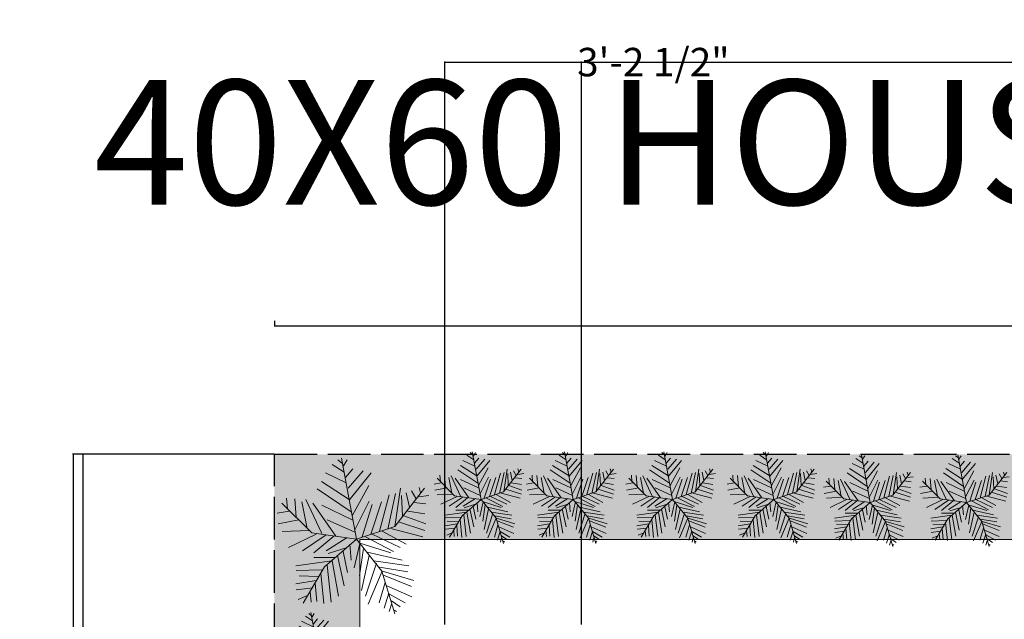
# Model space of a CAD drawing. Units: inches. Extents: x 853 to 1550, y 485 to 1596.
# Tile 14 of 18: x 862 to 1139, y 1428 to 1596. Entities that reach past the tile are written whole.
import ezdxf

# ---------------------------------------------------------------- set-up
doc = ezdxf.new("R2010")
doc.units = ezdxf.units.IN
doc.header["$MEASUREMENT"] = 0
doc.linetypes.add('ACAD_ISO02W100', pattern=[15, 12, -3])
for name, color, linetype, lineweight in [('A-ANNO-DIMS', 2, 'Continuous', 18), ('A-ANNO-TEXT', 250, 'Continuous', 25), ('C-PROP', 8, 'ACAD_ISO02W100', 25), ('L-PLNT-TREE', 106, 'Continuous', 13), ('lawn', 106, 'Continuous', 18)]:
    doc.layers.add(name, color=color, linetype=linetype, lineweight=lineweight)
doc.layers.add('L-PLNT-PATT', color=85, linetype='Continuous', lineweight=13, true_color=0x58ba48)
doc.styles.get("Standard").update_dxf_attribs({"font": 'arial.ttf'})
doc.dimstyles.get("Standard").update_dxf_attribs({"dimtxt": 8, "dimasz": 0.18, "dimexe": 0.18, "dimexo": 0.0625, "dimgap": 0.09, "dimtad": 0, "dimtih": 1, "dimtoh": 1, "dimzin": 0, "dimdsep": 46, "dimlunit": 3, "dimtxsty": 'Standard', "dimcen": 0.09, "dimadec": 0, "dimazin": 0, "dimtfac": 1, "dimtofl": 0, "dimtmove": 0, "dimatfit": 3, "dimfxl": 1, "dimtolj": 1, "dimtzin": 0, "dimarcsym": 0})

# ---------------------------------------------------------------- blocks, each defined once
blk = doc.blocks.new('*U18')
for p, q in [((-10.186, 53.64), (-13.084, 55.962)), ((0, 0), (-10.5, 57)), ((-9.099, 51.782), (-6.563, 55.962)), ((-8.737, 47.138), (-17.069, 52.711)), ((-7.65, 43.423), (-2.578, 49.46)), ((-7.288, 39.707), (-21.778, 46.673)), ((-5.839, 35.992), (4.667, 48.067)), ((-5.114, 27.632), (10.463, 46.673)), ((-3.665, 19.273), (-27.574, 35.527)), ((-5.114, 28.097), (-24.676, 40.636)), ((-2.941, 16.486), (8.652, 37.85)), ((27, 9), (48, 36)), ((27.127, 9.056), (31.112, 35.992)), ((44.153, 36.456), (45.239, 32.741)), ((-48.585, 21.131), (-49.309, 29.026)), ((-43.513, 28.561), (-42.427, 15.558)), ((-35.544, 28.097), (-24.314, 3.947)), ((16.259, 5.805), (23.142, 31.348)), ((22.055, 7.198), (27.489, 32.277)), ((31.836, 30.883), (32.561, 16.486)), ((35.096, 32.741), (37.27, 22.524)), ((38.719, 34.134), (41.979, 28.561)), ((43.791, 29.954), (51.036, 30.883)), ((-31.5, 4.5), (-52.5, 25.5)), ((-38.442, 26.239), (-34.819, 7.663)), ((-14.533, 2.09), (-30.834, 25.31)), ((-24.314, 23.917), (-2.941, 13.7)), ((-1.129, 6.734), (9.014, 26.704)), ((3.942, 1.625), (11.187, 24.381)), ((10.101, 3.483), (17.708, 26.239)), ((40.53, 25.775), (48.862, 24.846)), ((-47.498, 19.737), (-55.83, 18.344)), ((33.285, 16.486), (48.862, 10.913)), ((36.183, 19.737), (48.137, 17.88)), ((-40.615, 13.7), (-55.105, 10.913)), ((-20.691, 13.7), (-1.129, 4.876)), ((0, 0), (27, 9)), ((24.229, 7.663), (46.688, 1.625)), ((29.662, 12.307), (48.137, 6.269)), ((-33.37, 6.269), (-52.207, 5.34)), ((-28.299, 3.483), (-47.86, -5.805)), ((-21.416, 3.018), (-38.079, -8.128)), ((0, 0), (-31.5, 4.5)), ((-15.982, 2.09), (-30.11, -9.521)), ((0, 0), (-22.5, -19.5)), ((-6.563, 1.161), (-21.416, -8.128)), ((0, 0), (18, -22.5)), ((6.478, 1.625), (26.04, -8.592)), ((11.187, 3.483), (30.749, -5.805)), ((18.07, 5.805), (35.096, -3.483)), ((-6.563, -5.805), (-19.967, -9.985)), ((-4.752, -3.483), (-3.665, -14.629)), ((2.493, -3.019), (-1.491, -20.202)), ((1.769, -2.555), (24.229, -9.521)), ((5.029, -6.27), (2.131, -25.775)), ((-15.257, -12.772), (-30.11, -12.772)), ((-13.446, -11.378), (-8.737, -32.741)), ((-9.461, -8.592), (-6.201, -23.453)), ((9.014, -11.378), (3.58, -35.992)), ((7.565, -9.056), (32.198, -14.629)), ((-17.431, -15.094), (-42.789, -18.809)), ((-22.5, -19.5), (-37.5, -45)), ((-20.691, -18.345), (-17.793, -44.352)), ((-17.069, -15.094), (-12.721, -40.172)), ((14.085, -16.951), (6.478, -40.172)), ((12.274, -15.094), (36.907, -18.809)), ((16.259, -19.738), (36.183, -22.989)), ((-24.314, -21.596), (-42.427, -22.06)), ((-26.849, -26.24), (-40.253, -25.775)), ((-25.038, -23.918), (-22.865, -45.281)), ((18.07, -22.524), (8.289, -45.745)), ((18, -22.5), (27, -52.5)), ((18.433, -22.524), (40.53, -29.026)), ((19.157, -25.311), (38.719, -33.206)), ((-28.299, -29.026), (-42.789, -31.348)), ((-30.834, -34.135), (-42.427, -35.528)), ((-29.023, -30.884), (-27.936, -43.887)), ((20.244, -30.419), (15.897, -44.816)), ((21.331, -32.741), (39.081, -40.636)), ((-34.457, -39.708), (-40.978, -42.494)), ((-32.646, -36.921), (-31.921, -44.352)), ((22.78, -37.85), (19.519, -48.532)), ((22.78, -38.314), (34.372, -44.816)), ((24.591, -45.745), (23.142, -50.854)), ((24.591, -43.423), (30.749, -47.603)), ((26.764, -49.925), (28.213, -50.854))]:
    blk.add_line(p, q)
blk = doc.blocks.new('*D22')
at = {"layer": 'A-ANNO-DIMS', "color": 0, "lineweight": -2, "transparency": 16777216}
for p, q in [((933.94, 1511.65), (933.94, 1510.09)), ((1461.94, 1511.65), (1461.94, 1510.09)), ((934.12, 1510.27), (1190.9, 1510.27)), ((1461.76, 1510.27), (1204.98, 1510.27))]:
    blk.add_line(p, q, dxfattribs=at)
at = {"layer": 'A-ANNO-DIMS', "color": 0, "transparency": 16777216}
for points in [[(934.12, 1510.3), (934.12, 1510.24), (933.94, 1510.27)], [(1461.76, 1510.3), (1461.76, 1510.24), (1461.94, 1510.27)]]:
    blk.add_solid(points, dxfattribs=at)
at = {"layer": 'Defpoints', "color": 0, "transparency": 16777216}
for p in [(933.94, 1511.71), (1461.94, 1511.71), (1461.94, 1510.27)]:
    blk.add_point(p, dxfattribs=at)
at = {"layer": 'A-ANNO-DIMS', "color": 0, "transparency": 16777216, "insert": (1197.94, 1510.27), "char_height": 8, "attachment_point": 5}
blk.add_mtext("\\A1;40'", dxfattribs=at)
blk = doc.blocks.new('*D23')
at = {"layer": 'A-ANNO-DIMS', "color": 0, "lineweight": -2, "transparency": 16777216}
for p, q in [((879.97, 1474.13), (879.75, 1474.13)), ((879.93, 1473.95), (879.93, 1049.11)), ((879.93, 615.92), (879.93, 1040.76)), ((879.97, 615.74), (879.75, 615.74))]:
    blk.add_line(p, q, dxfattribs=at)
at = {"layer": 'A-ANNO-DIMS', "color": 0, "transparency": 16777216}
for points in [[(879.9, 1473.95), (879.96, 1473.95), (879.93, 1474.13)], [(879.9, 615.92), (879.96, 615.92), (879.93, 615.74)]]:
    blk.add_solid(points, dxfattribs=at)
at = {"layer": 'Defpoints', "color": 0, "transparency": 16777216}
for p in [(880.03, 1474.13), (879.93, 615.74), (880.03, 615.74)]:
    blk.add_point(p, dxfattribs=at)
at = {"layer": 'A-ANNO-DIMS', "color": 0, "transparency": 16777216, "insert": (879.93, 1044.94), "char_height": 8, "attachment_point": 5}
blk.add_mtext("\\A1;60'", dxfattribs=at)
blk = doc.blocks.new('*D69')
at = {"layer": 'A-ANNO-DIMS', "color": 0, "lineweight": -2, "transparency": 16777216}
for p, q in [((981.94, 1426.19), (981.94, 1584.65)), ((982.12, 1584.47), (1184.11, 1584.47)), ((1413.76, 1584.47), (1211.77, 1584.47)), ((1413.94, 1426.19), (1413.94, 1584.65))]:
    blk.add_line(p, q, dxfattribs=at)
at = {"layer": 'A-ANNO-DIMS', "color": 0, "transparency": 16777216}
for points in [[(982.12, 1584.5), (982.12, 1584.44), (981.94, 1584.47)], [(1413.76, 1584.5), (1413.76, 1584.44), (1413.94, 1584.47)]]:
    blk.add_solid(points, dxfattribs=at)
at = {"layer": 'Defpoints', "color": 0, "transparency": 16777216}
for p in [(1413.94, 1584.47), (981.94, 1426.13), (1413.94, 1426.13)]:
    blk.add_point(p, dxfattribs=at)
at = {"layer": 'A-ANNO-DIMS', "color": 0, "transparency": 16777216, "insert": (1197.94, 1584.47), "char_height": 8, "attachment_point": 5}
blk.add_mtext('\\A1;36\'-0"', dxfattribs=at)
blk = doc.blocks.new('*D71')
at = {"layer": 'A-ANNO-DIMS', "color": 0, "lineweight": -2, "transparency": 16777216}
for p, q in [((933.87, 1474.13), (877.09, 1474.13)), ((877.27, 1473.95), (877.27, 1015.66)), ((877.27, 549.16), (877.27, 1007.45)), ((933.87, 548.98), (877.09, 548.98))]:
    blk.add_line(p, q, dxfattribs=at)
at = {"layer": 'A-ANNO-DIMS', "color": 0, "transparency": 16777216}
for points in [[(877.24, 1473.95), (877.3, 1473.95), (877.27, 1474.13)], [(877.24, 549.16), (877.3, 549.16), (877.27, 548.98)]]:
    blk.add_solid(points, dxfattribs=at)
at = {"layer": 'Defpoints', "color": 0, "transparency": 16777216}
for p in [(877.27, 1474.13), (933.94, 1474.13), (933.94, 548.98)]:
    blk.add_point(p, dxfattribs=at)
at = {"layer": 'A-ANNO-DIMS', "color": 0, "transparency": 16777216, "insert": (877.27, 1011.55), "char_height": 8, "attachment_point": 5}
blk.add_mtext('\\A1;77\'-1"', dxfattribs=at)
blk = doc.blocks.new('*D82')
at = {"layer": 'A-ANNO-DIMS', "color": 0, "lineweight": -2, "transparency": 16777216}
for p, q in [((981.94, 1426.19), (981.94, 1584.65)), ((982.12, 1584.47), (1020.22, 1584.47)), ((1020.4, 1426.19), (1020.4, 1584.65)), ((1020.4, 1584.47), (1020.58, 1584.47))]:
    blk.add_line(p, q, dxfattribs=at)
at = {"layer": 'A-ANNO-DIMS', "color": 0, "transparency": 16777216}
for points in [[(982.12, 1584.5), (982.12, 1584.44), (981.94, 1584.47)], [(1020.22, 1584.5), (1020.22, 1584.44), (1020.4, 1584.47)]]:
    blk.add_solid(points, dxfattribs=at)
at = {"layer": 'Defpoints', "color": 0, "transparency": 16777216}
for p in [(1020.4, 1584.47), (981.94, 1426.13), (1020.4, 1426.13)]:
    blk.add_point(p, dxfattribs=at)
at = {"layer": 'A-ANNO-DIMS', "color": 0, "transparency": 16777216, "insert": (1040.62, 1584.47), "char_height": 8, "attachment_point": 5}
blk.add_mtext('\\A1;3\'-2 1/2"', dxfattribs=at)

msp = doc.modelspace()

# ---------------------------------------------------------------- hatches: boundary and pattern name
at = {"layer": 'L-PLNT-PATT'}
h = msp.add_hatch(color=256, dxfattribs=at)
h.dxf.hatch_style = 1
h.paths.add_polyline_path([(1461.937, 1474.129), (933.937, 1474.129), (933.937, 730.129), (933.937, 622.891), (941.686, 622.891), (941.686, 604.895), (957.937, 604.895), (957.937, 1450.129), (1437.937, 1450.129), (1437.937, 604.895), (1454.646, 604.895), (1454.646, 622.891), (1461.937, 622.891), (1461.937, 734.988)])

# ---------------------------------------------------------------- linework, layer by layer
at = {"layer": 'C-PROP'}
for p, q in [((933.937, 1474.129), (1461.937, 1474.129)), ((933.937, 730.129), (933.937, 1474.129))]:
    msp.add_line(p, q, dxfattribs=at)
at = {"layer": 'lawn'}
for p, q in [((957.937, 1450.129), (1437.937, 1450.129)), ((957.937, 765.455), (957.937, 1450.129))]:
    msp.add_line(p, q, dxfattribs=at)

# ---------------------------------------------------------------- block references
at = {"layer": 'L-PLNT-TREE'}
for p, xscale, yscale, zscale in [((957.009, 1450.196), 0.3996992985476591, 0.3996992985476591, 0.3996992985476591), ((992.091, 1461.393), 0.2357951711934384, 0.2357951711934384, 0.2357951711934384), ((1018.08, 1461.393), 0.2357951711934384, 0.2357951711934384, 0.2357951711934384), ((1046.047, 1461.393), 0.2357951711934384, 0.2357951711934384, 0.2357951711934384), ((1074.579, 1461.393), 0.2357951711934384, 0.2357951711934384, 0.2357951711934384), ((1101.699, 1460.518), 0.2357951711934384, 0.2357951711934384, 0.2357951711934384), ((1128.818, 1460.518), 0.2357951711934384, 0.2357951711934384, 0.2357951711934384), ((946.691, 1416.133), 0.2357951711934384, 0.2357951711934384, 0.2357951711934384)]:
    msp.add_blockref('*U18', p, dxfattribs=dict(at, xscale=xscale, yscale=yscale, zscale=zscale))

# ---------------------------------------------------------------- texts
at = {"layer": 'A-ANNO-TEXT'}
msp.add_text('40X60 HOUSE PLAN [4BHK]', height=35.05469, dxfattribs=at).set_placement((883.136, 1544.353))

# ---------------------------------------------------------------- dimensions: what is measured, and where the dimension line sits
at = {"layer": 'A-ANNO-DIMS'}
for base, p2, picture, middle in [((1020.402, 1584.468), (1020.402, 1426.129), '*D82', (1040.623, 1584.468)), ((1413.937, 1584.468), (1413.937, 1426.129), '*D69', (1197.937, 1584.468))]:
    dim = msp.add_linear_dim(base=base, p1=(981.937, 1426.129), p2=p2, dimstyle='Standard', override={"dimdec": 1, "dimlfac": 1, "dimrnd": 0, "dimzin": 1, "dimdsep": 46, "dimlunit": 4, "dimfrac": 2}, dxfattribs=at)
    dim.commit()
    dim.dimension.update_dxf_attribs({"geometry": picture, "text_midpoint": middle})
dim = msp.add_linear_dim(base=(1461.937, 1510.271), p1=(933.937, 1511.712), p2=(1461.937, 1511.712), text="40'", dimstyle='Standard', override={"dimclrd": 0, "dimclre": 0, "dimclrt": 0}, dxfattribs=at)
dim.commit()
dim.dimension.update_dxf_attribs({"geometry": '*D22', "text_midpoint": (1197.937, 1510.271)})
dim = msp.add_linear_dim(base=(877.2718, 1474.1293), p1=(933.9371, 548.9788), p2=(933.9371, 1474.1293), angle=90, dimstyle='Standard', override={"dimdec": 1, "dimlfac": 1, "dimrnd": 0, "dimzin": 1, "dimdsep": 46, "dimlunit": 4, "dimfrac": 2}, dxfattribs=at)
dim.commit()
dim.dimension.update_dxf_attribs({"geometry": '*D71', "text_midpoint": (877.2718, 1011.5541)})
dim = msp.add_linear_dim(base=(879.933, 615.743), p1=(880.035, 1474.129), p2=(880.035, 615.743), angle=90, text="60'", dimstyle='Standard', override={"dimclrd": 0, "dimclre": 0, "dimclrt": 0}, dxfattribs=at)
dim.commit()
dim.dimension.update_dxf_attribs({"geometry": '*D23', "text_midpoint": (879.933, 1044.936)})

doc.saveas('drawing.dxf')
